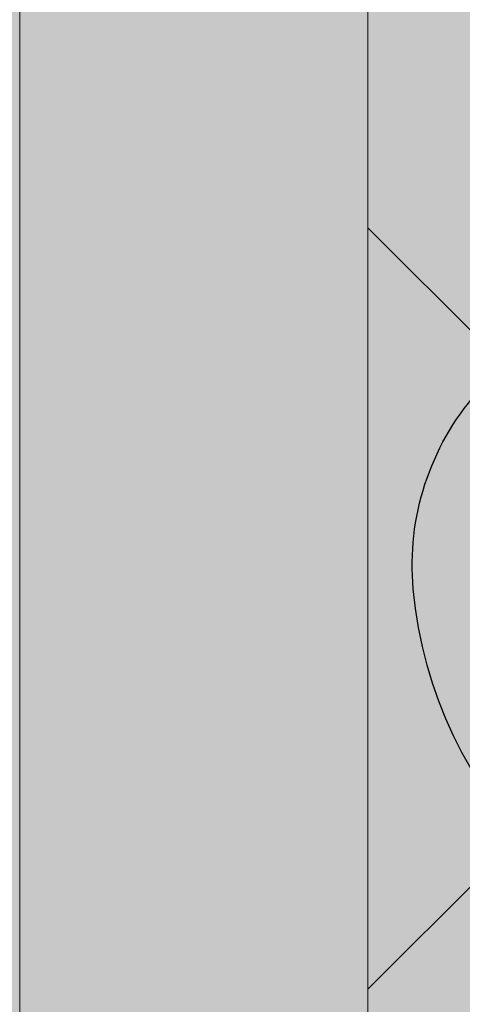
# Model space of a CAD drawing. Units: inches. Extents: x 844 to 2234, y 346 to 1084.
# Tile 70 of 93: x 1998.757 to 1999.568, y 692.525 to 694.327. Entities that reach past the tile are written whole.
import ezdxf

# ---------------------------------------------------------------- set-up
doc = ezdxf.new("R2010")
doc.units = ezdxf.units.IN
doc.header["$MEASUREMENT"] = 0
for name, color, linetype, lineweight in [('A-ANNO-DIMS', 2, 'Continuous', 18), ('furniture', 8, 'Continuous', 18), ('RA-AP-01$0$INT', 35, 'Continuous', 5)]:
    doc.layers.add(name, color=color, linetype=linetype, lineweight=lineweight)
doc.layers.add('RA-AP-01$0$FURN', color=3, linetype='Continuous')
doc.layers.add('RA-AP-01$0$WOOD', color=64, linetype='Continuous')
doc.styles.get("Standard").update_dxf_attribs({"font": 'arial.ttf'})
doc.dimstyles.get("Standard").update_dxf_attribs({"dimtxt": 6, "dimasz": 3, "dimexe": 0.18, "dimexo": 0.0625, "dimgap": 0.09, "dimtad": 0, "dimtih": 1, "dimtoh": 1, "dimdec": 1, "dimzin": 0, "dimdsep": 46, "dimlunit": 3, "dimtxsty": 'Standard', "dimblk": 'ARCHTICK', "dimcen": 0.09, "dimadec": 0, "dimazin": 0, "dimtfac": 1, "dimtdec": 1, "dimtofl": 0, "dimtmove": 0, "dimatfit": 3, "dimfxl": 1, "dimtolj": 1, "dimtzin": 0, "dimarcsym": 0})

# ---------------------------------------------------------------- blocks, each defined once
blk = doc.blocks.new('A$C18D01794')
at = {"layer": 'RA-AP-01$0$INT'}
h = blk.add_hatch(color=256, dxfattribs=at)
h.paths.add_polyline_path([(4.469348592586677, -7.07085414521094), (4.505206456958073, -7.03499628085108), (4.505206456958071, -7.106712009593861)])
h.paths.add_polyline_path([(4.455206456960671, -7.084996280832395), (4.476922185709333, -7.106712009588038), (4.433490728198045, -7.106712009588038)])
h.paths.add_polyline_path([(4.405206456958073, -7.034996280813718), (4.441064321339218, -7.070854145206393), (4.40520645695807, -7.106712009576003)])
h.paths.add_polyline_path([(4.425206456989053, -6.911460746921742), (4.455206456990736, -6.881460746929706), (4.485206456989055, -6.911460746937677), (4.48520645696979, -7.026712009590022), (4.455206456965227, -7.056712009584936), (4.425206456969784, -7.026712009579853)])
h.paths.add_polyline_path([(4.505206456958073, -6.831460746955388), (4.505206456958071, -6.903176475661116), (4.469348592616738, -6.867318611308251)])
h.paths.add_polyline_path([(4.425206456964688, -6.707925213036777), (4.455206456964794, -6.677925213027025), (4.485206456964689, -6.707925213017265), (4.485206456983951, -6.823176475683938), (4.455206456990736, -6.853176475686799), (4.425206456983956, -6.823176475689667)])
h.paths.add_polyline_path([(4.425206456974126, -6.504389679118949), (4.455206456959092, -6.474389679124341), (4.485206456974132, -6.504389679129721), (4.485206456993396, -6.619640941768059), (4.45520645699153, -6.649640941779566), (4.425206456993394, -6.619640941791077)])
h.paths.add_polyline_path([(4.46934859260189, -6.663783077416661), (4.505206456958071, -6.627925213048953), (4.505206456958073, -6.699640941761311)])
h.paths.add_polyline_path([(4.405206456958073, -6.627925213005104), (4.441064321354427, -6.663783077389926), (4.405206456958072, -6.699640941797813)])
h.paths.add_polyline_path([(4.405206456958072, -6.424389679139403), (4.441064321333084, -6.460247543502882), (4.405206456958072, -6.496105407889427)])
h.paths.add_polyline_path([(4.469348592580547, -6.460247543498336), (4.505206456958071, -6.424389679109282), (4.505206456958071, -6.496105407864332)])
h.paths.add_polyline_path([(4.425206456957888, -6.300854145208262), (4.45520645695415, -6.270854145221655), (4.485206456959507, -6.300854145217359), (4.48520645695824, -6.416105407863534), (4.455206456954537, -6.44610540787688), (4.425206456957888, -6.416105407889874)])
h.paths.add_polyline_path([(4.425206456957888, -6.226712009591025), (4.471064321332215, -6.226712009591025), (4.425206456957888, -6.272569873980103)])
h.paths.add_polyline_path([(4.499348592575121, -6.226712009591029), (4.636064321343707, -6.226712009591025), (4.666064321342317, -6.256712009589254), (4.636064321340932, -6.286712009591028), (4.499348592588945, -6.286712009591028), (4.469348592591685, -6.256712009584116)])
h.paths.add_polyline_path([(4.680206456964641, -6.270854145214393), (4.716064321337824, -6.306712009588038), (4.644348592591454, -6.306712009588038)])
h.paths.add_polyline_path([(4.644348592588108, -6.206712009588038), (4.716064321341167, -6.206712009588038), (4.680206456964637, -6.242569873964111)])
h.paths.add_polyline_path([(4.724348592586768, -6.226712009589824), (4.861064321340514, -6.226712009589824), (4.891064321340324, -6.256712009589255), (4.861064321340141, -6.286712009589827), (4.724348592587134, -6.286712009589821), (4.694348592586957, -6.256712009589254)])
h.paths.add_polyline_path([(4.905206456964143, -6.270854145212892), (4.941064321338827, -6.306712009588038), (4.869348592589457, -6.306712009588039)])
h.paths.add_polyline_path([(4.869348592586113, -6.206712009588038), (4.941064321342172, -6.206712009588038), (4.905206456964145, -6.242569873965612)])
h.paths.add_polyline_path([(4.949348592587774, -6.226712009589824), (5.086064321341521, -6.226712009589824), (5.116064321341329, -6.256712009589252), (5.08606432134115, -6.286712009589823), (4.949348592588145, -6.286712009589827), (4.919348592587961, -6.256712009589255)])
h.paths.add_polyline_path([(5.130206456963645, -6.270854145214393), (5.166064321336834, -6.306712009588038), (5.094348592590464, -6.306712009588038)])
h.paths.add_polyline_path([(5.094348592587119, -6.206712009588038), (5.166064321340178, -6.206712009588038), (5.130206456963651, -6.242569873964107)])
h.paths.add_polyline_path([(5.174348592584578, -6.226712009591027), (5.311064321353163, -6.226712009591027), (5.341064321336602, -6.256712009584116), (5.31106432133934, -6.286712009591028), (5.174348592587352, -6.286712009591028), (5.144348592585969, -6.256712009589254)])
h.paths.add_polyline_path([(5.325206456968778, -6.300854145217359), (5.355206456974136, -6.270854145221653), (5.385206456970396, -6.300854145208262), (5.385206456970396, -6.416105407889878), (5.355206456973747, -6.44610540787688), (5.325206456970044, -6.416105407863533)])
h.paths.add_polyline_path([(5.339348592596073, -6.226712009591029), (5.385206456970396, -6.226712009591025), (5.385206456970398, -6.272569873980105)])
h.paths.add_polyline_path([(5.325206456954155, -6.504389679129722), (5.355206456969194, -6.474389679124342), (5.38520645695416, -6.504389679118949), (5.385206456934896, -6.619640941791077), (5.355206456936758, -6.649640941779564), (5.325206456934888, -6.619640941768057)])
h.paths.add_polyline_path([(5.305206456958072, -6.424389679097139), (5.341064321347739, -6.460247543498338), (5.305206456958072, -6.496105407876472)])
h.paths.add_polyline_path([(5.369348592595204, -6.460247543502882), (5.40520645695807, -6.42438967915155), (5.405206456958072, -6.496105407877278)])
h.paths.add_polyline_path([(5.405206456958072, -6.627925213017245), (5.405206456958072, -6.69964094178567), (5.369348592573857, -6.663783077389926)])
h.paths.add_polyline_path([(5.305206456958072, -6.62792521303681), (5.341064321326393, -6.663783077416663), (5.305206456958072, -6.69964094177345)])
h.paths.add_polyline_path([(5.325206456963599, -6.707925213017267), (5.355206456963494, -6.677925213027021), (5.385206456963598, -6.707925213036775), (5.385206456944334, -6.823176475689665), (5.355206456937552, -6.853176475686797), (5.325206456944333, -6.823176475683936)])
h.paths.add_polyline_path([(5.305206456958072, -6.831460746943246), (5.341064321311551, -6.867318611308252), (5.305206456958072, -6.903176475673257)])
h.paths.add_polyline_path([(5.325206456939231, -6.911460746937672), (5.355206456937552, -6.881460746929707), (5.385206456939235, -6.911460746921742), (5.385206456958502, -7.026712009579853), (5.355206456963061, -7.056712009584934), (5.3252064569585, -7.026712009590026)])
h.paths.add_polyline_path([(5.404581768715993, -6.832085435167151, 0.001217816984214), (5.405206456958072, -6.832312009593747), (5.405206456958072, -6.90317647569123), (5.369348592563558, -6.867318611308251)])
h.paths.add_polyline_path([(5.36934859258907, -7.070854145206393), (5.40520645695807, -7.034996280825861), (5.405206456958072, -7.106712009563858)])
h.paths.add_polyline_path([(5.355206456967613, -7.084996280832394), (5.376922185730239, -7.106712009588038), (5.333490728218953, -7.106712009588036)])
h.paths.add_polyline_path([(5.30520645695807, -7.034996280838937), (5.341064321341609, -7.070854145210942), (5.305206456958074, -7.106712009606006)])
h = blk.add_hatch(color=256, dxfattribs=at)
h.paths.add_polyline_path([(4.505206456958071, -6.627925213048953), (4.46934859260189, -6.663783077416663), (4.505206456958071, -6.699640941761309), (4.505206456958071, -6.831460746955389), (4.469348592616735, -6.867318611308252), (4.505206456958071, -6.903176475661112), (4.505206456958071, -7.03499628085108), (4.469348592586679, -7.070854145210939), (4.505206456952245, -7.106712009588038), (4.476922185709333, -7.106712009588038), (4.455206456960671, -7.084996280832395), (4.433490728198047, -7.106712009588038), (4.405206456946033, -7.10671200958804), (4.441064321339216, -7.070854145206393), (4.40520645695807, -7.034996280813718), (4.405206456958072, -6.903176475703379), (4.441064321364728, -6.867318611308251), (4.40520645695807, -6.83146074691313), (4.40520645695807, -6.699640941797813), (4.441064321354429, -6.663783077389924), (4.405206456958072, -6.627925213005102), (4.405206456958072, -6.496105407889425), (4.441064321333084, -6.460247543502882), (4.405206456958072, -6.424389679139403), (4.405206456958072, -6.206712009588038), (4.644348592588106, -6.206712009588038), (4.680206456964639, -6.242569873964107), (4.716064321341165, -6.206712009588038), (4.869348592586113, -6.206712009588038), (4.905206456964143, -6.24256987396561), (4.941064321342174, -6.206712009588038), (5.094348592587118, -6.206712009588038), (5.130206456963649, -6.242569873964107), (5.166064321340178, -6.206712009588038), (5.405206456958072, -6.206712009588038), (5.405206456958072, -6.42438967915155), (5.369348592595202, -6.46024754350288), (5.40520645695807, -6.49610540787728), (5.40520645695807, -6.627925213017247), (5.369348592573859, -6.663783077389926), (5.40520645695807, -6.699640941785666), (5.40520645695807, -6.831460746925273), (5.36934859256356, -6.867318611308252), (5.405206456958072, -6.90317647569123), (5.405206456958072, -7.034996280825859), (5.369348592589068, -7.070854145206395), (5.405206456982249, -7.106712009588038), (5.376922185730244, -7.106712009588038), (5.355206456967613, -7.084996280832397), (5.333490728218955, -7.106712009588036), (5.305206456976043, -7.106712009588035), (5.341064321341609, -7.07085414521094), (5.305206456958072, -7.034996280838935), (5.305206456958072, -6.90317647567326), (5.34106432131155, -6.867318611308252), (5.305206456958072, -6.831460746943244), (5.30520645695807, -6.699640941773452), (5.341064321326395, -6.663783077416663), (5.305206456958072, -6.627925213036814), (5.305206456958072, -6.496105407876472), (5.341064321347738, -6.46024754349834), (5.305206456958072, -6.424389679097137), (5.30520645695807, -6.306712009588038), (5.166064321336834, -6.306712009588038), (5.130206456963647, -6.270854145214393), (5.094348592590464, -6.306712009588038), (4.941064321338827, -6.306712009588036), (4.905206456964145, -6.270854145212892), (4.869348592589459, -6.306712009588038), (4.716064321337822, -6.306712009588036), (4.680206456964641, -6.270854145214393), (4.644348592591453, -6.306712009588038), (4.505206456958071, -6.306712009588038), (4.505206456958071, -6.424389679109282), (4.469348592580545, -6.460247543498338), (4.505206456958071, -6.496105407864328)])
h.paths.add_polyline_path([(4.485206456974132, -6.504389679129722), (4.45520645695909, -6.474389679124341), (4.425206456974128, -6.504389679118945), (4.425206456993394, -6.619640941791079), (4.45520645699153, -6.649640941779566), (4.485206456993396, -6.619640941768059)], flags=16)
h.paths.add_polyline_path([(4.455206456954537, -6.44610540787688), (4.485206456958242, -6.416105407863534), (4.48520645695951, -6.30085414521736), (4.45520645695415, -6.270854145221653), (4.425206456957888, -6.300854145208264), (4.425206456957888, -6.41610540788988)], flags=16)
h.paths.add_polyline_path([(4.455206456964794, -6.677925213027025), (4.42520645696469, -6.707925213036777), (4.425206456983954, -6.82317647568967), (4.455206456990734, -6.853176475686797), (4.485206456983953, -6.823176475683936), (4.485206456964687, -6.707925213017265)], flags=16)
h.paths.add_polyline_path([(4.499348592588947, -6.286712009591028), (4.636064321340932, -6.286712009591028), (4.666064321342317, -6.256712009589254), (4.636064321343707, -6.226712009591027), (4.499348592575121, -6.226712009591029), (4.469348592591685, -6.256712009584118)], flags=16)
h.paths.add_polyline_path([(4.425206456957888, -6.272569873980103), (4.471064321332215, -6.226712009591025), (4.425206456957888, -6.226712009591025)], flags=16)
h.paths.add_polyline_path([(4.455206456990734, -6.881460746929709), (4.425206456989053, -6.91146074692174), (4.425206456969784, -7.026712009579853), (4.455206456965226, -7.056712009584932), (4.485206456969787, -7.026712009590026), (4.485206456989053, -6.911460746937672)], flags=16)
h.paths.add_polyline_path([(4.72434859258714, -6.286712009589821), (4.861064321340141, -6.286712009589829), (4.891064321340324, -6.256712009589254), (4.861064321340513, -6.226712009589823), (4.724348592586768, -6.226712009589823), (4.694348592586956, -6.256712009589254)], flags=16)
h.paths.add_polyline_path([(4.919348592587961, -6.256712009589254), (4.949348592588145, -6.286712009589827), (5.08606432134115, -6.286712009589823), (5.116064321341327, -6.256712009589254), (5.086064321341519, -6.226712009589824), (4.949348592587774, -6.226712009589824)], flags=16)
h.paths.add_polyline_path([(5.144348592585967, -6.256712009589254), (5.174348592587358, -6.286712009591028), (5.311064321339338, -6.286712009591028), (5.3410643213366, -6.256712009584118), (5.311064321353163, -6.226712009591029), (5.174348592584576, -6.226712009591027)], flags=16)
h.paths.add_polyline_path([(5.32520645693489, -6.619640941768055), (5.355206456936755, -6.649640941779566), (5.385206456934894, -6.619640941791079), (5.38520645695416, -6.504389679118949), (5.355206456969194, -6.474389679124341), (5.325206456954153, -6.504389679129724)], flags=16)
h.paths.add_polyline_path([(5.325206456970042, -6.416105407863534), (5.355206456973747, -6.44610540787688), (5.385206456970398, -6.416105407889876), (5.385206456970398, -6.30085414520826), (5.355206456974136, -6.270854145221653), (5.325206456968778, -6.30085414521736)], flags=16)
h.paths.add_polyline_path([(5.325206456963599, -6.707925213017265), (5.325206456944333, -6.823176475683936), (5.355206456937552, -6.853176475686797), (5.385206456944332, -6.823176475689667), (5.385206456963596, -6.707925213036773), (5.355206456963492, -6.677925213027027)], flags=16)
h.paths.add_polyline_path([(5.32520645693923, -6.911460746937674), (5.3252064569585, -7.026712009590026), (5.355206456963062, -7.056712009584934), (5.3852064569585, -7.026712009579853), (5.385206456939234, -6.911460746921738), (5.355206456937552, -6.881460746929707)], flags=16)
h.paths.add_polyline_path([(5.339348592596071, -6.226712009591029), (5.385206456970398, -6.272569873980103), (5.385206456970396, -6.226712009591027)], flags=16)
blk.add_hatch(color=256, dxfattribs=at).paths.add_polyline_path([(4.505206456958071, -6.306712009588038), (5.305206456958072, -6.306712009588038), (5.305206456958072, -7.106712009588038), (5.255206456951893, -7.10671200958804), (5.25520645694868, -6.356712009605972), (4.555206456959269, -6.356712009587461), (4.555206456956052, -7.106712009588038), (4.505206456958073, -7.106712009588038)])
h = blk.add_hatch(color=256, dxfattribs=at)
h.paths.add_polyline_path([(4.585917135068448, -6.356712009588273), (4.614201406330596, -6.356712009589021), (4.668846067270487, -6.411356670531338), (4.723490728212344, -6.356712009591912), (4.771774999457151, -6.35671200959319), (4.826419660396886, -6.411356670535356), (4.862780050090322, -6.374996280843536), (4.844495778842715, -6.356712009595112), (4.862780050090411, -6.356712009595595), (4.905206456960182, -6.399138416468211), (4.947632863832445, -6.356712009597838), (4.965917135079675, -6.356712009598322), (4.947632863831759, -6.374996280845421), (4.983993253523576, -6.411356670538857), (5.038637914464627, -6.356712009600247), (5.08692218571208, -6.356712009601523), (5.141566846649976, -6.411356670541852), (5.196211507589851, -6.356712009604411), (5.224495778822615, -6.356712009605161), (4.905206456953975, -6.676001331473793)])
h.paths.add_polyline_path([(4.895206456956031, -6.637717060225675), (4.895206456958921, -6.528427738347902), (4.840561796018589, -6.583072399285802)], flags=16)
h.paths.add_polyline_path([(4.915206456955638, -6.637717060226121), (4.969851117895509, -6.583072399288678), (4.915206456957609, -6.528427738348344)], flags=16)
h.paths.add_polyline_path([(4.826419660395175, -6.568930263661755), (4.881064321335613, -6.514285602723745), (4.771774999456703, -6.514285602720857)], flags=16)
h.paths.add_polyline_path([(4.983993253519558, -6.568930263665262), (5.038637914460456, -6.514285602726792), (4.929348592581548, -6.514285602724816)], flags=16)
h.paths.add_polyline_path([(4.881064321336025, -6.494285602723742), (4.826419660397532, -6.439640941782821), (4.771774999457062, -6.494285602720859)], flags=16)
h.paths.add_polyline_path([(4.929348592582019, -6.494285602724817), (5.038637914460982, -6.494285602726792), (4.983993253522945, -6.439640941786327)], flags=16)
h.paths.add_polyline_path([(4.895206456960191, -6.480143467100443), (4.895206456962115, -6.407422687715913), (4.876922185715016, -6.389138416467584), (4.840561796021581, -6.425498806159401)], flags=16)
h.paths.add_polyline_path([(4.915206456958487, -6.480143467100889), (4.969851117899527, -6.425498806162279), (4.933490728206909, -6.389138416468043), (4.9152064569598, -6.40742268771434)], flags=16)
h.paths.add_polyline_path([(4.757632863832376, -6.480143467096812), (4.812277524772842, -6.425498806158772), (4.757632863834348, -6.370854145217844)], flags=16)
h.paths.add_polyline_path([(4.737632863832376, -6.480143467096286), (4.737632863834348, -6.370854145217375), (4.682988202893906, -6.425498806155385)], flags=16)
h.paths.add_polyline_path([(5.05278005008503, -6.480143467103376), (5.052780050087917, -6.370854145224413), (4.998135389146995, -6.425498806162908)], flags=16)
h.paths.add_polyline_path([(5.072780050085024, -6.480143467103744), (5.127424711025931, -6.42549880616527), (5.072780050087916, -6.370854145224832)], flags=16)
h.paths.add_polyline_path([(4.935917135072783, -6.706712009592292), (5.255206456948811, -6.387422687716309), (5.255206456948932, -6.415706958964177), (5.200561796010279, -6.470351619902839), (5.255206456949403, -6.524996280841948), (5.25520645694961, -6.5732805520894), (5.200561796009787, -6.627925213029239), (5.236922185702417, -6.664285602721864), (5.255206456949919, -6.646001331474357), (5.255206456949998, -6.664285602721898), (5.212780050078687, -6.706712009592262), (5.25520645695036, -6.749138416463932), (5.255206456950438, -6.767422687711313), (5.236922185702424, -6.749138416463297), (5.200561796009796, -6.785498806155928), (5.255206456950753, -6.840143467096874), (5.25520645695096, -6.888427738341682), (5.200561796010322, -6.943072399282328), (5.255206456951428, -6.997717060223427), (5.255206456951547, -7.026001331471006)])
h.paths.add_polyline_path([(5.042988202883395, -6.785498806155427), (5.097632863823085, -6.840143467095101), (5.097632863822622, -6.730854145216193)], flags=16)
h.paths.add_polyline_path([(5.028846067259663, -6.771356670531693), (5.083490728198774, -6.716712009592573), (4.974201406321001, -6.716712009593042)], flags=16)
h.paths.add_polyline_path([(5.117632863823087, -6.840143467095186), (5.172277524762331, -6.785498806155926), (5.11763286382262, -6.730854145216225)], flags=16)
h.paths.add_polyline_path([(5.08349072819877, -6.696712009593886), (5.028846067259652, -6.642067348654775), (4.974201406320998, -6.696712009593438)], flags=16)
h.paths.add_polyline_path([(5.131774999446817, -6.854285602718917), (5.186419660386065, -6.799640941779662), (5.241064321325782, -6.854285602719365)], flags=17)
h.paths.add_polyline_path([(5.131774999446228, -6.716712009592374), (5.186419660386065, -6.771356670532194), (5.222780050079488, -6.734996280838764), (5.204495778832781, -6.716712009592063)], flags=16)
h.paths.add_polyline_path([(5.097632863822613, -6.682569873970264), (5.097632863823061, -6.573280552091354), (5.042988202883383, -6.627925213031044)], flags=16)
h.paths.add_polyline_path([(5.131774999446899, -6.874285602718915), (5.241064321325809, -6.874285602719364), (5.186419660386591, -6.928930263658598)], flags=17)
h.paths.add_polyline_path([(5.131774999446226, -6.696712009594078), (5.204495778830767, -6.696712009594374), (5.22278005007868, -6.67842773834687), (5.186419660386049, -6.642067348654249)], flags=16)
h.paths.add_polyline_path([(5.11763286382262, -6.682569873970225), (5.17227752476232, -6.627925213030515), (5.117632863823064, -6.573280552091267)], flags=16)
h.paths.add_polyline_path([(5.186419660386069, -6.613783077405491), (5.241064321325754, -6.559138416465795), (5.131774999446791, -6.559138416466263)], flags=16)
h.paths.add_polyline_path([(5.131774999446872, -6.539138416466263), (5.24106432132578, -6.539138416465794), (5.186419660386554, -6.484493755526573)], flags=16)
h.paths.add_polyline_path([(5.255206456951811, -7.08742268770861), (5.255206456951895, -7.106712009588038), (4.555206456956052, -7.106712009588038), (4.555206456956136, -7.087422687708617), (4.905206456953973, -6.737422687710788)])
h.paths.add_polyline_path([(4.983993253513404, -6.8444937555241), (4.92934859257295, -6.899138416462108), (5.03863791445186, -6.899138416465014)], flags=16)
h.paths.add_polyline_path([(4.969851117889988, -6.83035161990006), (4.915206456952556, -6.775706958960171), (4.915206456949648, -6.884996280837944)], flags=16)
h.paths.add_polyline_path([(4.929348592572535, -6.919138416462105), (4.983993253511019, -6.973783077403037), (5.038637914451496, -6.919138416465012)], flags=16)
h.paths.add_polyline_path([(5.052780050074912, -6.93328055208906), (4.998135389134438, -6.987925213027088), (5.052780050072919, -7.042569873968025)], flags=16)
h.paths.add_polyline_path([(5.07278005007491, -6.933280552089588), (5.072780050072918, -7.042569873968497), (5.127424711013374, -6.987925213030498)], flags=16)
h.paths.add_polyline_path([(4.89520645695295, -6.775706958959721), (4.840561796013067, -6.830351619897157), (4.895206456950961, -6.884996280837494)], flags=16)
h.paths.add_polyline_path([(4.915206456948365, -6.933280552085403), (4.915206456946434, -7.006001331471951), (4.933490728192729, -7.024285602719066), (4.969851117886972, -6.987925213026453)], flags=16)
h.paths.add_polyline_path([(4.881064321327021, -6.899138416461022), (4.82641966038902, -6.84449375552057), (4.771774999448108, -6.899138416459029)], flags=16)
h.paths.add_polyline_path([(4.895206456950073, -6.933280552084951), (4.840561796009022, -6.987925213023558), (4.876922185700835, -7.024285602716997), (4.895206456948749, -7.006001331469487)], flags=16)
h.paths.add_polyline_path([(4.983993253510392, -7.0020673486505), (4.947632863816944, -7.038427738342319), (4.965917135064043, -7.05671200959023), (5.038637914448995, -7.056712009591555)], flags=16)
h.paths.add_polyline_path([(4.881064321326543, -6.91913841646102), (4.771774999447578, -6.919138416459031), (4.826419660385607, -6.973783077399508)], flags=16)
h.paths.add_polyline_path([(4.905206456946447, -7.014285602717636), (4.862780050074785, -7.056712009588352), (4.947632863816685, -7.056712009589775)], flags=16)
h.paths.add_polyline_path([(5.14156684663679, -7.002067348654549), (5.086922185696452, -7.056712009592438), (5.196211507574223, -7.056712009594425)], flags=16)
h.paths.add_polyline_path([(4.8264196603837, -7.002067348646972), (4.771774999442643, -7.056712009585575), (4.8444957788276, -7.056712009587508), (4.862780050075511, -7.038427738340416)], flags=16)
h.paths.add_polyline_path([(4.812277524760289, -6.98792521302292), (4.757632863822258, -6.933280552082447), (4.757632863819352, -7.042569873961408)], flags=16)
h.paths.add_polyline_path([(4.73763286382226, -6.933280552082079), (4.682988202881349, -6.987925213020536), (4.737632863819352, -7.04256987396099)], flags=16)
h.paths.add_polyline_path([(4.723490728195188, -7.056712009584289), (4.668846067257299, -7.002067348643949), (4.614201406317417, -7.056712009581383)], flags=16)
h.paths.add_polyline_path([(4.597632863829262, -6.706712009592262), (4.555206456957951, -6.664285602721896), (4.555206456958029, -6.646001331474357), (4.573490728205535, -6.664285602721864), (4.609851117898167, -6.627925213029238), (4.555206456958338, -6.573280552089402), (4.555206456958546, -6.524996280841952), (4.60985111789767, -6.470351619902839), (4.555206456959015, -6.415706958964177), (4.555206456959138, -6.387422687716309), (4.874495778835167, -6.70671200959229), (4.5552064569564, -7.026001331471015), (4.555206456956523, -6.997717060223433), (4.609851117897629, -6.94307239928233), (4.555206456956988, -6.888427738341681), (4.555206456957198, -6.840143467096881), (4.609851117898153, -6.78549880615593), (4.573490728205528, -6.749138416463297), (4.555206456957507, -6.76742268771132), (4.555206456957585, -6.749138416463933)])
h.paths.add_polyline_path([(4.712780050085332, -6.730854145216195), (4.712780050084863, -6.840143467095105), (4.767424711024555, -6.785498806155427)], flags=16)
h.paths.add_polyline_path([(4.726922185709173, -6.716712009592573), (4.781566846648288, -6.771356670531693), (4.836211507586949, -6.716712009593043)], flags=16)
h.paths.add_polyline_path([(4.692780050085327, -6.730854145216225), (4.638135389145619, -6.785498806155928), (4.692780050084865, -6.840143467095185)], flags=16)
h.paths.add_polyline_path([(4.726922185709182, -6.696712009593886), (4.836211507586949, -6.696712009593436), (4.7815668466483, -6.642067348654773)], flags=16)
h.paths.add_polyline_path([(4.678637914461726, -6.71671200959237), (4.605917135075169, -6.716712009592063), (4.587632863828464, -6.734996280838766), (4.623993253521887, -6.771356670532195)], flags=16)
h.paths.add_polyline_path([(4.712780050085336, -6.68256987397026), (4.767424711024568, -6.627925213031042), (4.71278005008489, -6.573280552091352)], flags=16)
h.paths.add_polyline_path([(4.678637914461726, -6.696712009594076), (4.623993253521899, -6.642067348654247), (4.587632863829271, -6.67842773834687), (4.605917135077185, -6.696712009594376)], flags=16)
h.paths.add_polyline_path([(4.692780050085336, -6.682569873970228), (4.692780050084889, -6.573280552091267), (4.638135389145632, -6.627925213030515)], flags=16)
h.paths.add_polyline_path([(4.623993253521885, -6.799640941779662), (4.678637914461131, -6.854285602718915), (4.56934859258217, -6.854285602719365)], flags=17)
h.paths.add_polyline_path([(4.623993253521901, -6.613783077405509), (4.678637914461158, -6.559138416466263), (4.569348592582195, -6.559138416465795)], flags=16)
h.paths.add_polyline_path([(4.678637914461051, -6.874285602718915), (4.623993253521361, -6.928930263658598), (4.569348592582143, -6.874285602719364)], flags=17)
h.paths.add_polyline_path([(4.678637914461076, -6.539138416466263), (4.623993253521399, -6.484493755526573), (4.569348592582167, -6.539138416465796)], flags=16)
h = blk.add_hatch(color=256, dxfattribs=at)
h.paths.add_polyline_path([(5.028846067259997, -6.642067348655121), (4.974201406321342, -6.696712009593783), (5.083490728199115, -6.69671200959423)])
h.paths.add_polyline_path([(4.974201406321344, -6.716712009593388), (5.028846067260004, -6.771356670532039), (5.083490728199117, -6.716712009592919)])
h.paths.add_polyline_path([(5.042988202883738, -6.785498806155768), (5.097632863823428, -6.840143467095449), (5.097632863822963, -6.73085414521654)])
h.paths.add_polyline_path([(5.117632863822961, -6.730854145216568), (5.117632863823428, -6.840143467095531), (5.172277524762674, -6.785498806156272)])
h.paths.add_polyline_path([(5.131774999446572, -6.716712009592718), (5.186419660386406, -6.77135667053254), (5.222780050079831, -6.734996280839116), (5.204495778833122, -6.716712009592409)])
h.paths.add_polyline_path([(5.236922185702764, -6.749138416463644), (5.200561796010139, -6.785498806156274), (5.255206456949971, -6.840143467096101), (5.255206456950271, -6.76742268771115)])
h.paths.add_polyline_path([(5.186419660386412, -6.799640941780006), (5.131774999447164, -6.854285602719262), (5.241064321326123, -6.854285602719711)])
h.paths.add_polyline_path([(5.131774999447238, -6.874285602719261), (5.186419660386934, -6.928930263658944), (5.241064321326153, -6.874285602719709)])
h.paths.add_polyline_path([(5.200561796010663, -6.943072399282675), (5.255206456949324, -6.997717060221329), (5.255206456949777, -6.888427738343558)])
h.paths.add_polyline_path([(5.21278005007903, -6.706712009592607), (5.255206456950223, -6.749138416463798), (5.255206456950696, -6.664285602721891)])
h.paths.add_polyline_path([(5.13177499944657, -6.696712009594424), (5.204495778831106, -6.696712009594723), (5.222780050079024, -6.678427738347219), (5.186419660386397, -6.642067348654592)])
h.paths.add_polyline_path([(5.117632863823405, -6.573280552091611), (5.117632863822955, -6.682569873970578), (5.172277524762665, -6.627925213030859)])
h.paths.add_polyline_path([(5.042988202883727, -6.627925213031387), (5.097632863822957, -6.682569873970603), (5.097632863823407, -6.573280552091697)])
h.paths.add_polyline_path([(5.131774999447135, -6.559138416466609), (5.186419660386394, -6.613783077405857), (5.241064321326097, -6.559138416466144)])
h.paths.add_polyline_path([(5.200561796010128, -6.627925213029584), (5.236922185702758, -6.664285602722211), (5.255206456950264, -6.646001331474705), (5.255206456949948, -6.573280552089752)])
h.paths.add_polyline_path([(5.186419660386895, -6.484493755526919), (5.131774999447213, -6.539138416466609), (5.241064321326127, -6.539138416466142)])
h.paths.add_polyline_path([(5.200561796010624, -6.470351619903183), (5.255206456949745, -6.524996280842298), (5.255206456949276, -6.415706958964523)])
for p, q in [((5.255206456951895, -7.106712009588038), (5.255206456948681, -6.356712009605972)), ((5.255206456948934, -6.415706958964177), (5.200561796010281, -6.470351619902839)), ((5.255206456949399, -6.524996280841946), (5.200561796010281, -6.470351619902839))]:
    blk.add_line(p, q, dxfattribs=at)
blk.add_lwpolyline([(5.305206456958072, -7.106712009588038), (5.305206456958072, -6.306712009588038), (4.505206456958071, -6.306712009588038), (4.505206456958071, -7.106712009588038)], dxfattribs=at)
blk = doc.blocks.new('A$C32926AE1')
at = {"layer": 'RA-AP-01$0$WOOD'}
h = blk.add_hatch(color=256, dxfattribs=at)
h.dxf.hatch_style = 1
h.paths.add_polyline_path([(5.157430609644524, 4.573483066760929, -0.1009492694046607), (5.155401577623758, 4.593365984175333, -0.1842662638101597), (5.172249623284174, 4.638795604568598, 0.2056608120311276), (5.179560981299304, 4.661316324430096, 0.3614336704623542), (5.134352340494423, 4.706524965234944, 0.2056608120311297), (5.111831620632933, 4.699213607219793, -0.1842662638101113), (5.066402000239693, 4.682365561559342, -0.1055311479399994), (5.045656153913092, 4.68467289944697, 0.1567636581983829), (4.763886414745334, 4.684672899446966, -0.1055311479399895), (4.743140568418733, 4.68236556155934, -0.1842662638100833), (4.6977109480255, 4.69921360721979, 0.2056608120302612), (4.675190228164109, 4.706524965234949, 0.3614336704708441), (4.629981587358889, 4.66131632442871, 0.2056608120245944), (4.637292945374126, 4.638795604567974, -0.1842662638101024), (4.654140991034615, 4.59336598417475, -0.1009492694055169), (4.652111959013835, 4.573483066760181, 0.021410119221476), (4.629748025606143, 4.156712009541676, 0.0214101192214795), (4.652111959013809, 3.739940952323101, -0.1009492694059586), (4.654140991034615, 3.720058034908448, -0.1842662638100975), (4.637292945374126, 3.674628414515226, 0.2056608120245705), (4.629981587358889, 3.652107694654492, 0.3614336704708879), (4.675190228164113, 3.606899053848249, 0.2056608120302384), (4.697710948025501, 3.614210411863408, -0.1842662638100995), (4.743140568418738, 3.63105845752386, -0.1055311479402541), (4.763886414745388, 3.628751119636215, 0.1567636581983776), (5.045656153913137, 3.628751119636244, -0.1055311479397538), (5.066402000239692, 3.631058457523857, -0.1842662638101067), (5.111831620632931, 3.614210411863407, 0.2056608120310924), (5.134352340494417, 3.606899053848256, 0.3614336704624001), (5.179560981299307, 3.652107694653103, 0.2056608120311314), (5.172249623284175, 3.6746284145146, -0.1842662638101402), (5.155401577623758, 3.72005803490786, -0.1009492694051366), (5.15743060964455, 3.739940952322354, 0.0214101192215073), (5.179794543052287, 4.156712009541468, 0.0214101192215252)])
h.paths.add_polyline_path([(4.639748609479751, 4.156712009541513, 0.0213537860821624), (4.661970494867118, 3.741887061152232, -0.094075836301374), (4.664143710413708, 3.7196126951003, -0.1824818158568985), (4.644813765429836, 3.668037719127816, 0.2056608120245319), (4.639939526753007, 3.653023905887301, 0.3614336704710246), (4.676106439397173, 3.616856993242342, 0.2056608120302234), (4.691120252638095, 3.621731231919122, -0.1824818158602558), (4.742695228611606, 3.641061176902986, -0.1029891339458722), (4.766991894714349, 3.638256818950944, 0.156709409989566), (5.042550673941472, 3.638256818950105, -0.102989133958497), (5.066847340047078, 3.641061176902949, -0.1824818158594995), (5.118422316020358, 3.621731231919103, 0.2056608120311416), (5.133436129261316, 3.616856993242346, 0.3614336704621468), (5.169603041905217, 3.653023905886178, 0.2056608120310986), (5.164728803228477, 3.668037719127177, -0.1824818158565612), (5.145398858244737, 3.719612695099578, -0.0940758363009313), (5.147572073791232, 3.741887061151398, 0.0213537860822023), (5.169793959178681, 4.156712009541451, 0.0213537860822226), (5.147572073791203, 4.571536957931898, -0.0940758363005034), (5.145398858244737, 4.59381132398362, -0.1824818158565587), (5.164728803228476, 4.645386299956021, 0.2056608120311045), (5.169603041905216, 4.66040011319702, 0.3614336704621845), (5.133436129261313, 4.696567025840856, 0.2056608120310773), (5.118422316020359, 4.691692787164098, -0.182481815859508), (5.066847340047078, 4.67236284218025, -0.1029891339584606), (5.04255067394148, 4.675167200133092, 0.156709409989566), (4.766991894714357, 4.675167200132257, -0.1029891339458842), (4.742695228611611, 4.672362842180213, -0.1824818158602725), (4.691120252638095, 4.691692787164077, 0.2056608120302152), (4.676106439397174, 4.696567025840858, 0.3614336704710363), (4.639939526753005, 4.660400113195899, 0.2056608120245495), (4.644813765429837, 4.645386299955384, -0.1824818158568934), (4.664143710413708, 4.593811323982902, -0.0940758363009187), (4.661970494867149, 4.571536957931074, 0.021353786082177)], flags=16)
h.paths.add_polyline_path([(5.129794543052235, 4.432167055276933, -0.0141661062790638), (5.130152669293814, 4.156927903047693, -0.0141661062790647), (5.129794543052234, 3.881688750818433, -0.0785247771143638), (5.10979738006795, 3.755143611847103, 0.0945969212073497), (5.105408519571111, 3.717898134952927, 0.1043170707844957), (5.116074640131521, 3.670385395016088, 0.1043170707864965), (5.068561900193738, 3.681051515576561, 0.09459692119553), (5.031316423304057, 3.676662655080835, -0.1580239521427272), (4.778226145355827, 3.676662655080367, 0.0945969211986668), (4.740980668464973, 3.681051515576592, 0.1043170707882822), (4.693467928526415, 3.670385395015844, 0.1043170707867916), (4.704134049087309, 3.717898134953662, 0.0945969211972894), (4.69974518859162, 3.755143611844042, -0.0785247771163196), (4.679748025606343, 3.881688750818406, -0.0141661062790663), (4.679389899364763, 4.156927903047693, -0.0141661062790672), (4.679748025606343, 4.432167055276998, -0.0785247771163064), (4.699745188591625, 4.55871219425134, 0.094596921197333), (4.704134049087308, 4.595957671141738, 0.1043170707867205), (4.693467928526416, 4.643470411079523, 0.1043170707882628), (4.740980668464965, 4.632804290518776, 0.0945969211988114), (4.778226145355874, 4.637193151015016, -0.158023952142669), (5.031316423304015, 4.637193151014546, 0.0945969211956361), (5.068561900193736, 4.632804290518806, 0.1043170707864979), (5.11607464013152, 4.643470411079278, 0.1043170707844617), (5.105408519571112, 4.595957671142455, 0.0945969212074597), (5.109797380067959, 4.558712194248236, -0.0785247771143467)], flags=0)
h.paths.add_polyline_path([(5.119794532311105, 4.432259799204851, -0.0142000800617244), (5.120156169157484, 4.156927903047701, -0.0142000800617277), (5.119794532311105, 3.881596006890482, -0.0784894509520253), (5.100273383573699, 3.758192358677797, 0.0940138827242913), (5.095413455884425, 3.717477693979438, 0.0606271852308753), (5.099615656341024, 3.686844378806616, 0.0606271852322524), (5.068982341167493, 3.691046579263239, 0.0940138827010453), (5.028267676478798, 3.686186651576848, -0.1580706864508061), (4.781274892180912, 3.686186651576435, 0.0940138827026903), (4.740560227491556, 3.691046579263279, 0.0606271852339895), (4.709926912317155, 3.686844378806508, 0.0606271852329405), (4.714129112773991, 3.717477693980356, 0.094013882701304), (4.709269185087677, 3.758192358669163, -0.0784894509577193), (4.689748036347473, 3.881596006890469, -0.014200080061729), (4.689386399501094, 4.156927903047709, -0.0142000800617217), (4.689748036347473, 4.432259799204808, -0.078489450957724), (4.709269185087651, 4.555663447426125, 0.0940138827014585), (4.714129112773992, 4.596378112114996, 0.0606271852329731), (4.709926912317154, 4.62701142728886, 0.0606271852340196), (4.74056022749157, 4.622809226832087, 0.0940138827024997), (4.781274892180847, 4.627669154518912, -0.1580706864508359), (5.028267676478777, 4.627669154518526, 0.0940138827010946), (5.068982341167492, 4.622809226832129, 0.060627185232254), (5.099615656341024, 4.627011427288751, 0.0606271852308727), (5.095413455884425, 4.59637811211593, 0.0940138827241088), (5.100273383573675, 4.555663447417647, -0.0784894509520978)], flags=0)
h.paths.add_polyline_path([(5.06978912287499, 4.430218106756144, -0.014241683694547), (5.070173729147532, 4.156927903047672, -0.0142416836945458), (5.06978912287499, 3.883637699339223, -0.0800609523125196), (5.052662118612511, 3.773463122773442, 0.0526421978001116), (5.04590916754064, 3.740550867606997, 0.0526421977992423), (5.012996912374707, 3.73379791653534, -0.1583028414718258), (4.796545656286308, 3.73379791653451, 0.0526421978034211), (4.763633401117837, 3.740550867607021, 0.0526421978018622), (4.756880450045755, 3.773463122774558, -0.0800609523117106), (4.739753445783639, 3.883637699339268, -0.0142416836945435), (4.739368839511098, 4.156927903047671, -0.0142416836945477), (4.739753445783639, 4.430218106756155, -0.0800609523116345), (4.75688045004574, 4.540392683320762, 0.052642197801941), (4.763633401117837, 4.573304938488346, 0.0526421978035071), (4.796545656286361, 4.580057889560873, -0.1583028414717561), (5.012996912374669, 4.580057889560039, 0.0526421977993048), (5.04590916754064, 4.57330493848837, 0.0526421978002057), (5.052662118612529, 4.540392683321868, -0.080060952312477)], flags=0)
h.paths.add_polyline_path([(5.049789715110557, 4.43038092723357, -0.0143097550741839), (5.05018085590259, 4.156927903047715, -0.0143097550741854), (5.049789715110558, 3.883474878861827, -0.0800685599149176), (5.03362098255317, 3.779581877367999, 0.0306258898956367), (5.028241146483733, 3.758218888663947, 0.0306258898977031), (5.006878157778253, 3.75283905259408, -0.1583983521624096), (4.802664410878162, 3.752839052594731, 0.0306258898946014), (4.781301422174808, 3.758218888663924, 0.0306258898967912), (4.775921586105202, 3.779581877368794, -0.080068559914251), (4.759752853548071, 3.883474878861786, -0.0143097550741854), (4.759361712756037, 4.156927903047671, -0.0143097550741854), (4.759752853548071, 4.430380927233557, -0.0800685599142479), (4.775921586105193, 4.534273928726546, 0.0306258898968306), (4.781301422174808, 4.555636917431444, 0.0306258898945754), (4.802664410878143, 4.561016753500631, -0.1583983521624168), (5.006878157778244, 4.561016753501291, 0.0306258898977177), (5.028241146483733, 4.555636917431421, 0.0306258898958182), (5.03362098255321, 4.534273928727244, -0.080068559914796)], flags=0)
h.paths.add_polyline_path([(4.999766070382627, 4.428171244713864, -0.0143443147609634), (5.000198441819402, 4.156927903047689, -0.0143443147609612), (4.999766070382627, 3.885684561381556, -0.0784641635803329), (4.987356730658798, 3.799103304488872, -0.1506053783831347), (4.822185837999821, 3.79910330448882, -0.0784641635803318), (4.809776498276007, 3.885684561381509, -0.014344314760963), (4.809344126839227, 4.156927903047677, -0.0143443147609645), (4.809776498276007, 4.428171244713873, -0.0784641635803192), (4.822185837999822, 4.514752501606549, -0.1506053783831338), (4.987356730658798, 4.514752501606494, -0.078464163580285)], flags=0)
h.paths.add_polyline_path([(4.979755254238824, 4.42764379880488, -0.0143772539198268), (4.980205517789977, 4.156927903047693, -0.0143772539198275), (4.979755254238824, 3.886212007290489, -0.0689242507424422), (4.971183264704897, 3.815276770442801, -0.1296645318904179), (4.838359303953726, 3.815276770442746, -0.0689242507424186), (4.829787314419809, 3.886212007290419, -0.0143772539198292), (4.829337050868653, 4.156927903047653, -0.0143772539198325), (4.829787314419809, 4.427643798804946, -0.0689242507424211), (4.838359303953725, 4.498579035652621, -0.1296645318904187), (4.971183264704897, 4.498579035652565, -0.0689242507424401)], flags=0)
for centre, radius, start, end in [((5.149687163117039, 3.654856328352376), 0.0300000000000001, 354.7431240045364, 41.22894907959901), ((5.129771284329024, 3.656688750818544), 0.0499999999998358, 275.2568759945053, 354.7431240047624)]:
    blk.add_arc(centre, radius, start, end, dxfattribs=at)
blk = doc.blocks.new('A$C5D2F253E')
at = {"layer": 'RA-AP-01$0$FURN', "xscale": -0.7999999999883585, "yscale": 0.7999999999883585, "zscale": 0.8, "rotation": 90}
blk.add_blockref('A$C18D01794', (-5.687757199772477, 4.75791982714071), dxfattribs=at)
at = {"layer": 'RA-AP-01$0$WOOD', "rotation": 270}
blk.add_blockref('A$C32926AE1', (-4.161339601644158, 5.73852594588169), dxfattribs=at)
blk = doc.blocks.new('_ArchTick')
at = {"color": 0, "linetype": 'ByBlock', "const_width": 0.15}
blk.add_lwpolyline([(-0.5, -0.5), (0.5, 0.5)], dxfattribs=at)
blk = doc.blocks.new('*D121')
at = {"layer": 'A-ANNO-DIMS', "color": 0, "lineweight": -2, "transparency": 16777216}
for p, q in [((2030.271987351997, 734.262611118704), (2040.245275089302, 734.262611118704)), ((2040.065275089302, 734.262611118704), (2040.065275089302, 704.6043509484256)), ((2040.065275089302, 668.557359536674), (2040.065275089302, 698.2156197069523)), ((2030.271987351997, 668.557359536674), (2040.245275089302, 668.557359536674))]:
    blk.add_line(p, q, dxfattribs=at)
at = {"layer": 'Defpoints', "color": 0, "transparency": 16777216}
for p in [(2030.209487351997, 734.262611118704), (2040.065275089302, 734.262611118704), (2030.209487351997, 668.557359536674)]:
    blk.add_point(p, dxfattribs=at)
at = {"layer": 'A-ANNO-DIMS', "color": 0, "lineweight": -2, "transparency": 16777216, "xscale": 3, "yscale": 3, "zscale": 3}
for p, rotation in [((2040.065275089302, 734.262611118704), 90), ((2040.065275089302, 668.557359536674), 270)]:
    blk.add_blockref('_ArchTick', p, dxfattribs=dict(at, rotation=rotation))
at = {"layer": 'A-ANNO-DIMS', "color": 0, "transparency": 16777216, "insert": (2040.065275089302, 701.4099853276883), "char_height": 6, "attachment_point": 5}
blk.add_mtext('\\A1;LOUNGE SET 5\'-5 1/2" TYP.', dxfattribs=at)

msp = doc.modelspace()

# ---------------------------------------------------------------- block references
at = {"layer": 'furniture', "xscale": -15.94108302203742, "yscale": 15.94108302203742, "zscale": 15.94108302203742, "rotation": 270}
msp.add_blockref('A$C5D2F253E', (1990.567271852805, 701.4028671565849), dxfattribs=at)

# ---------------------------------------------------------------- dimensions: what is measured, and where the dimension line sits
at = {"layer": 'A-ANNO-DIMS'}
dim = msp.add_linear_dim(base=(2040.065275089302, 734.262611118704), p1=(2030.209487351996, 668.5573595366737), p2=(2030.209487351996, 734.2626111187037), angle=90, text='LOUNGE SET <> TYP.', dimstyle='Standard', override={"dimdec": 1, "dimlfac": 1, "dimrnd": 0, "dimzin": 1, "dimdsep": 46, "dimlunit": 4, "dimfrac": 2}, dxfattribs=at)
dim.commit()
dim.dimension.update_dxf_attribs({"geometry": '*D121', "text_midpoint": (2040.065275089302, 701.4099853276883)})

doc.saveas('drawing.dxf')
